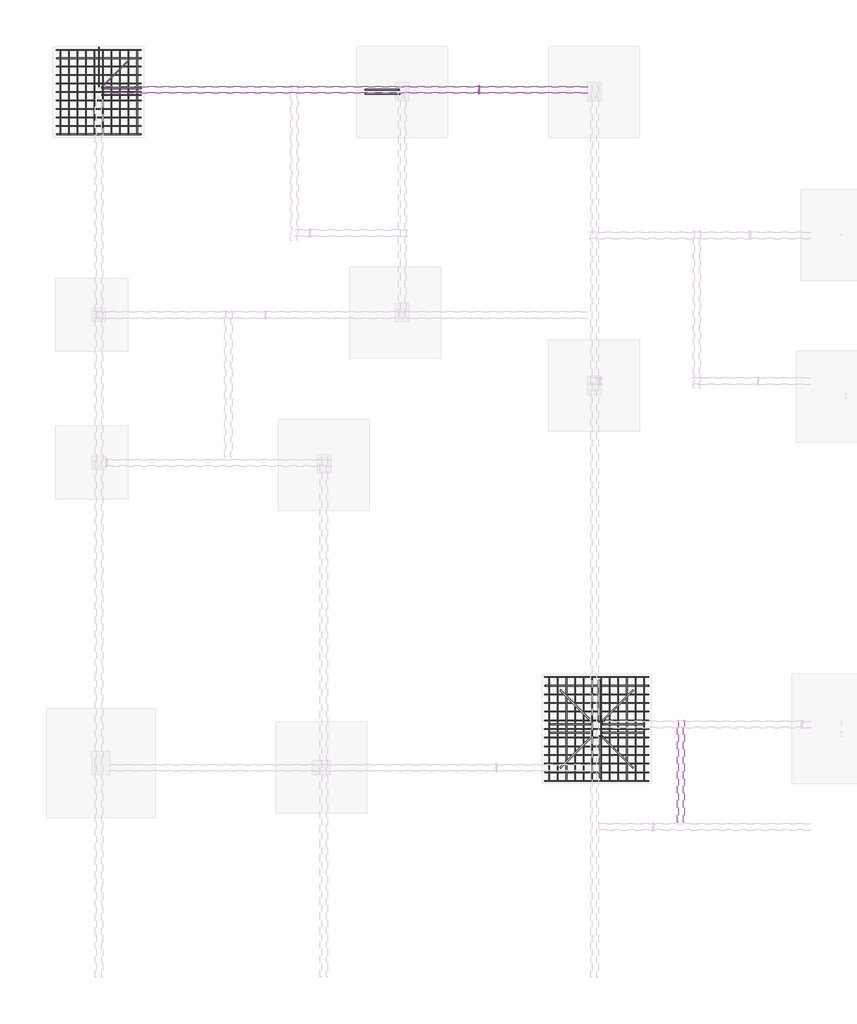
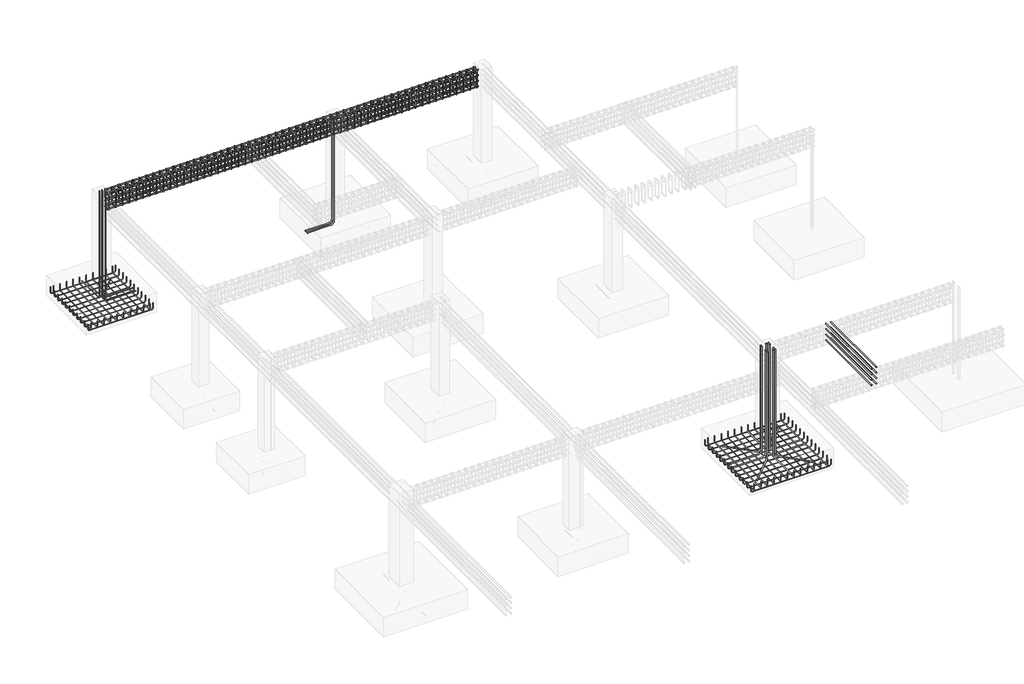
# One storey, part 7 of 10: 24 reinforcing bars.
"""IFC4 building model written with IfcOpenShell, lengths in millimetres."""

from ifc_helpers import new_model, si_unit, point, frame, origin, place, context, project, spatial, polyline, circle_curve, trimmed, segment, composite_curve, source, transform, mapped, element, save
from ifc_brep_helpers import swept_disk

model = new_model("IFC4")

# Units and contexts
model_context = context("Model", 3, world=origin())
ifc_project = project(units=[si_unit("LENGTHUNIT", "METRE", prefix="MILLI")], contexts=[model_context])

# Site, building, storey
site = spatial("IfcSite", under=ifc_project)
building = spatial("IfcBuilding", under=site)
storey = spatial("IfcBuildingStorey", under=building, Elevation=-2133.6)

# Reinforcing bars
placement = place(None, origin())
reinforcing_bar_shape = source(origin(), model_context, "Body", "SolidModel", [
    swept_disk(composite_curve([segment(polyline([(-4228.0164362, 12858.0219177, -2383.6), (-4228.0164362, 12858.0219177, -2494.1)]), True, "CONTINUOUS"), segment(trimmed(circle_curve(frame((-4262.7664362, 12858.0219177, -2494.1), z_axis=(0.0, 1.0, 0.0), x_axis=(34.75, 0.0, 0.0)), 34.75), [point((-4228.0164362, 12858.0219177, -2494.1))], [point((-4262.7664362, 12858.0219177, -2528.85))], True, "CARTESIAN"), True, "CONTINUOUS"), segment(polyline([(-4262.7664362, 12858.0219177, -2528.85), (-5607.7664362, 12858.0219177, -2528.85)]), True, "CONTINUOUS"), segment(trimmed(circle_curve(frame((-5607.7664362, 12858.0219177, -2494.1), z_axis=(0.0, 1.0, 0.0), x_axis=(0.0, 0.0, -34.75)), 34.75), [point((-5607.7664362, 12858.0219177, -2528.85))], [point((-5642.5164362, 12858.0219177, -2494.1))], True, "CARTESIAN"), True, "CONTINUOUS"), segment(polyline([(-5642.5164362, 12858.0219177, -2494.1), (-5642.5164362, 12858.0219177, -2383.6)]), True, "CONTINUOUS")], self_intersect=False), 4.75),
])
element("IfcReinforcingBar", 1, at=placement, inside=storey, context=model_context, shape_type="MappedRepresentation", body=[
    mapped(reinforcing_bar_shape, transform((0.0, 0.0, 0.0), x_axis=(1.0, 0.0, 0.0), y_axis=(0.0, 1.0, 0.0), z_axis=(0.0, 0.0, 1.0))),
    mapped(reinforcing_bar_shape, transform((0.0, -141.45, 0.0), x_axis=(1.0, 0.0, 0.0), y_axis=(0.0, 1.0, 0.0), z_axis=(0.0, 0.0, 1.0))),
    mapped(reinforcing_bar_shape, transform((0.0, -282.9, 0.0), x_axis=(1.0, 0.0, 0.0), y_axis=(0.0, 1.0, 0.0), z_axis=(0.0, 0.0, 1.0))),
    mapped(reinforcing_bar_shape, transform((0.0, -424.35, 0.0), x_axis=(1.0, 0.0, 0.0), y_axis=(0.0, 1.0, 0.0), z_axis=(0.0, 0.0, 1.0))),
    mapped(reinforcing_bar_shape, transform((0.0, -565.8, 0.0), x_axis=(1.0, 0.0, 0.0), y_axis=(0.0, 1.0, 0.0), z_axis=(0.0, 0.0, 1.0))),
    mapped(reinforcing_bar_shape, transform((0.0, -707.25, 0.0), x_axis=(1.0, 0.0, 0.0), y_axis=(0.0, 1.0, 0.0), z_axis=(0.0, 0.0, 1.0))),
    mapped(reinforcing_bar_shape, transform((0.0, -848.7, 0.0), x_axis=(1.0, 0.0, 0.0), y_axis=(0.0, 1.0, 0.0), z_axis=(0.0, 0.0, 1.0))),
    mapped(reinforcing_bar_shape, transform((0.0, -990.15, 0.0), x_axis=(1.0, 0.0, 0.0), y_axis=(0.0, 1.0, 0.0), z_axis=(0.0, 0.0, 1.0))),
    mapped(reinforcing_bar_shape, transform((0.0, -1131.6, 0.0), x_axis=(1.0, 0.0, 0.0), y_axis=(0.0, 1.0, 0.0), z_axis=(0.0, 0.0, 1.0))),
    mapped(reinforcing_bar_shape, transform((0.0, -1273.05, 0.0), x_axis=(1.0, 0.0, 0.0), y_axis=(0.0, 1.0, 0.0), z_axis=(0.0, 0.0, 1.0))),
    mapped(reinforcing_bar_shape, transform((0.0, -1414.5, 0.0), x_axis=(1.0, 0.0, 0.0), y_axis=(0.0, 1.0, 0.0), z_axis=(0.0, 0.0, 1.0))),
])
reinforcing_bar_2_shape = source(origin(), model_context, "Body", "SolidModel", [
    swept_disk(composite_curve([segment(polyline([(-4292.9743867, 11443.5219177, -2379.223371), (-4292.9743867, 11443.5219177, -2489.723371)]), True, "CONTINUOUS"), segment(trimmed(circle_curve(frame((-4292.9743867, 11478.2719177, -2489.723371), z_axis=(1.0, 0.0, 0.0), x_axis=(0.0, -34.75, 0.0)), 34.75), [point((-4292.9743867, 11443.5219177, -2489.723371))], [point((-4292.9743867, 11478.2719177, -2524.473371))], True, "CARTESIAN"), True, "CONTINUOUS"), segment(polyline([(-4292.9743867, 11478.2719177, -2524.473371), (-4292.9743867, 12823.2719177, -2524.473371)]), True, "CONTINUOUS"), segment(trimmed(circle_curve(frame((-4292.9743867, 12823.2719177, -2489.723371), z_axis=(1.0, 0.0, 0.0), x_axis=(0.0, 0.0, -34.75)), 34.75), [point((-4292.9743867, 12823.2719177, -2524.473371))], [point((-4292.9743867, 12858.0219177, -2489.723371))], True, "CARTESIAN"), True, "CONTINUOUS"), segment(polyline([(-4292.9743867, 12858.0219177, -2489.723371), (-4292.9743867, 12858.0219177, -2379.223371)]), True, "CONTINUOUS")], self_intersect=False), 4.75),
])
element("IfcReinforcingBar", 2, at=placement, inside=storey, context=model_context, shape_type="MappedRepresentation", body=[
    mapped(reinforcing_bar_2_shape, transform((0.0, 0.0, 0.0), x_axis=(1.0, 0.0, 0.0), y_axis=(0.0, 1.0, 0.0), z_axis=(0.0, 0.0, 1.0))),
    mapped(reinforcing_bar_2_shape, transform((-143.1506365, 0.0, 0.0), x_axis=(1.0, 0.0, 0.0), y_axis=(0.0, 1.0, 0.0), z_axis=(0.0, 0.0, 1.0))),
    mapped(reinforcing_bar_2_shape, transform((-286.301273, 0.0, 0.0), x_axis=(1.0, 0.0, 0.0), y_axis=(0.0, 1.0, 0.0), z_axis=(0.0, 0.0, 1.0))),
    mapped(reinforcing_bar_2_shape, transform((-429.4519095, 0.0, 0.0), x_axis=(1.0, 0.0, 0.0), y_axis=(0.0, 1.0, 0.0), z_axis=(0.0, 0.0, 1.0))),
    mapped(reinforcing_bar_2_shape, transform((-572.602546, 0.0, 0.0), x_axis=(1.0, 0.0, 0.0), y_axis=(0.0, 1.0, 0.0), z_axis=(0.0, 0.0, 1.0))),
    mapped(reinforcing_bar_2_shape, transform((-715.7531825, 0.0, 0.0), x_axis=(1.0, 0.0, 0.0), y_axis=(0.0, 1.0, 0.0), z_axis=(0.0, 0.0, 1.0))),
    mapped(reinforcing_bar_2_shape, transform((-858.903819, 0.0, 0.0), x_axis=(1.0, 0.0, 0.0), y_axis=(0.0, 1.0, 0.0), z_axis=(0.0, 0.0, 1.0))),
    mapped(reinforcing_bar_2_shape, transform((-1002.0544555, 0.0, 0.0), x_axis=(1.0, 0.0, 0.0), y_axis=(0.0, 1.0, 0.0), z_axis=(0.0, 0.0, 1.0))),
    mapped(reinforcing_bar_2_shape, transform((-1145.205092, 0.0, 0.0), x_axis=(1.0, 0.0, 0.0), y_axis=(0.0, 1.0, 0.0), z_axis=(0.0, 0.0, 1.0))),
    mapped(reinforcing_bar_2_shape, transform((-1288.3557284, 0.0, 0.0), x_axis=(1.0, 0.0, 0.0), y_axis=(0.0, 1.0, 0.0), z_axis=(0.0, 0.0, 1.0))),
])
reinforcing_bar_3_shape = source(origin(), model_context, "Body", "SolidModel", [
    swept_disk(composite_curve([segment(polyline([(4278.2835638, 2353.1839177, -2393.6), (4278.2835638, 2353.1839177, -2504.1)]), True, "CONTINUOUS"), segment(trimmed(circle_curve(frame((4243.5335638, 2353.1839177, -2504.1), z_axis=(0.0, 1.0, 0.0), x_axis=(34.75, 0.0, 0.0)), 34.75), [point((4278.2835638, 2353.1839177, -2504.1))], [point((4243.5335638, 2353.1839177, -2538.85))], True, "CARTESIAN"), True, "CONTINUOUS"), segment(polyline([(4243.5335638, 2353.1839177, -2538.85), (2573.7335638, 2353.1839177, -2538.85)]), True, "CONTINUOUS"), segment(trimmed(circle_curve(frame((2573.7335638, 2353.1839177, -2504.1), z_axis=(0.0, 1.0, 0.0), x_axis=(0.0, 0.0, -34.75)), 34.75), [point((2573.7335638, 2353.1839177, -2538.85))], [point((2538.9835638, 2353.1839177, -2504.1))], True, "CARTESIAN"), True, "CONTINUOUS"), segment(polyline([(2538.9835638, 2353.1839177, -2504.1), (2538.9835638, 2353.1839177, -2393.6)]), True, "CONTINUOUS")], self_intersect=False), 4.75),
])
element("IfcReinforcingBar", 3, at=placement, inside=storey, context=model_context, shape_type="MappedRepresentation", body=[
    mapped(reinforcing_bar_3_shape, transform((0.0, 0.0, 0.0), x_axis=(1.0, 0.0, 0.0), y_axis=(0.0, 1.0, 0.0), z_axis=(0.0, 0.0, 1.0))),
    mapped(reinforcing_bar_3_shape, transform((0.0, -144.9416667, 0.0), x_axis=(1.0, 0.0, 0.0), y_axis=(0.0, 1.0, 0.0), z_axis=(0.0, 0.0, 1.0))),
    mapped(reinforcing_bar_3_shape, transform((0.0, -289.8833333, 0.0), x_axis=(1.0, 0.0, 0.0), y_axis=(0.0, 1.0, 0.0), z_axis=(0.0, 0.0, 1.0))),
    mapped(reinforcing_bar_3_shape, transform((0.0, -434.825, 0.0), x_axis=(1.0, 0.0, 0.0), y_axis=(0.0, 1.0, 0.0), z_axis=(0.0, 0.0, 1.0))),
    mapped(reinforcing_bar_3_shape, transform((0.0, -579.7666667, 0.0), x_axis=(1.0, 0.0, 0.0), y_axis=(0.0, 1.0, 0.0), z_axis=(0.0, 0.0, 1.0))),
    mapped(reinforcing_bar_3_shape, transform((0.0, -724.7083333, 0.0), x_axis=(1.0, 0.0, 0.0), y_axis=(0.0, 1.0, 0.0), z_axis=(0.0, 0.0, 1.0))),
    mapped(reinforcing_bar_3_shape, transform((0.0, -869.65, 0.0), x_axis=(1.0, 0.0, 0.0), y_axis=(0.0, 1.0, 0.0), z_axis=(0.0, 0.0, 1.0))),
    mapped(reinforcing_bar_3_shape, transform((0.0, -1014.5916667, 0.0), x_axis=(1.0, 0.0, 0.0), y_axis=(0.0, 1.0, 0.0), z_axis=(0.0, 0.0, 1.0))),
    mapped(reinforcing_bar_3_shape, transform((0.0, -1159.5333333, 0.0), x_axis=(1.0, 0.0, 0.0), y_axis=(0.0, 1.0, 0.0), z_axis=(0.0, 0.0, 1.0))),
    mapped(reinforcing_bar_3_shape, transform((0.0, -1304.475, 0.0), x_axis=(1.0, 0.0, 0.0), y_axis=(0.0, 1.0, 0.0), z_axis=(0.0, 0.0, 1.0))),
    mapped(reinforcing_bar_3_shape, transform((0.0, -1449.4166667, 0.0), x_axis=(1.0, 0.0, 0.0), y_axis=(0.0, 1.0, 0.0), z_axis=(0.0, 0.0, 1.0))),
    mapped(reinforcing_bar_3_shape, transform((0.0, -1594.3583333, 0.0), x_axis=(1.0, 0.0, 0.0), y_axis=(0.0, 1.0, 0.0), z_axis=(0.0, 0.0, 1.0))),
    mapped(reinforcing_bar_3_shape, transform((0.0, -1739.3, 0.0), x_axis=(1.0, 0.0, 0.0), y_axis=(0.0, 1.0, 0.0), z_axis=(0.0, 0.0, 1.0))),
])
reinforcing_bar_4_shape = source(origin(), model_context, "Body", "SolidModel", [
    swept_disk(composite_curve([segment(polyline([(4203.3256133, 613.8839177, -2379.223371), (4203.3256133, 613.8839177, -2489.723371)]), True, "CONTINUOUS"), segment(trimmed(circle_curve(frame((4203.3256133, 648.6339177, -2489.723371), z_axis=(1.0, 0.0, 0.0), x_axis=(0.0, -34.75, 0.0)), 34.75), [point((4203.3256133, 613.8839177, -2489.723371))], [point((4203.3256133, 648.6339177, -2524.473371))], True, "CARTESIAN"), True, "CONTINUOUS"), segment(polyline([(4203.3256133, 648.6339177, -2524.473371), (4203.3256133, 2318.4339177, -2524.473371)]), True, "CONTINUOUS"), segment(trimmed(circle_curve(frame((4203.3256133, 2318.4339177, -2489.723371), z_axis=(1.0, 0.0, 0.0), x_axis=(0.0, 0.0, -34.75)), 34.75), [point((4203.3256133, 2318.4339177, -2524.473371))], [point((4203.3256133, 2353.1839177, -2489.723371))], True, "CARTESIAN"), True, "CONTINUOUS"), segment(polyline([(4203.3256133, 2353.1839177, -2489.723371), (4203.3256133, 2353.1839177, -2379.223371)]), True, "CONTINUOUS")], self_intersect=False), 4.75),
])
element("IfcReinforcingBar", 4, at=placement, inside=storey, context=model_context, shape_type="MappedRepresentation", body=[
    mapped(reinforcing_bar_4_shape, transform((0.0, 0.0, 0.0), x_axis=(1.0, 0.0, 0.0), y_axis=(0.0, 1.0, 0.0), z_axis=(0.0, 0.0, 1.0))),
    mapped(reinforcing_bar_4_shape, transform((-144.8323389, 0.0, 0.0), x_axis=(1.0, 0.0, 0.0), y_axis=(0.0, 1.0, 0.0), z_axis=(0.0, 0.0, 1.0))),
    mapped(reinforcing_bar_4_shape, transform((-289.6646779, 0.0, 0.0), x_axis=(1.0, 0.0, 0.0), y_axis=(0.0, 1.0, 0.0), z_axis=(0.0, 0.0, 1.0))),
    mapped(reinforcing_bar_4_shape, transform((-434.4970168, 0.0, 0.0), x_axis=(1.0, 0.0, 0.0), y_axis=(0.0, 1.0, 0.0), z_axis=(0.0, 0.0, 1.0))),
    mapped(reinforcing_bar_4_shape, transform((-579.3293558, 0.0, 0.0), x_axis=(1.0, 0.0, 0.0), y_axis=(0.0, 1.0, 0.0), z_axis=(0.0, 0.0, 1.0))),
    mapped(reinforcing_bar_4_shape, transform((-724.1616947, 0.0, 0.0), x_axis=(1.0, 0.0, 0.0), y_axis=(0.0, 1.0, 0.0), z_axis=(0.0, 0.0, 1.0))),
    mapped(reinforcing_bar_4_shape, transform((-868.9940337, 0.0, 0.0), x_axis=(1.0, 0.0, 0.0), y_axis=(0.0, 1.0, 0.0), z_axis=(0.0, 0.0, 1.0))),
    mapped(reinforcing_bar_4_shape, transform((-1013.8263726, 0.0, 0.0), x_axis=(1.0, 0.0, 0.0), y_axis=(0.0, 1.0, 0.0), z_axis=(0.0, 0.0, 1.0))),
    mapped(reinforcing_bar_4_shape, transform((-1158.6587116, 0.0, 0.0), x_axis=(1.0, 0.0, 0.0), y_axis=(0.0, 1.0, 0.0), z_axis=(0.0, 0.0, 1.0))),
    mapped(reinforcing_bar_4_shape, transform((-1303.4910505, 0.0, 0.0), x_axis=(1.0, 0.0, 0.0), y_axis=(0.0, 1.0, 0.0), z_axis=(0.0, 0.0, 1.0))),
    mapped(reinforcing_bar_4_shape, transform((-1448.3233895, 0.0, 0.0), x_axis=(1.0, 0.0, 0.0), y_axis=(0.0, 1.0, 0.0), z_axis=(0.0, 0.0, 1.0))),
    mapped(reinforcing_bar_4_shape, transform((-1593.1557284, 0.0, 0.0), x_axis=(1.0, 0.0, 0.0), y_axis=(0.0, 1.0, 0.0), z_axis=(0.0, 0.0, 1.0))),
])
element("IfcReinforcingBar", 5, at=placement, inside=storey, context=model_context, shape_type="SolidModel", body=[
    swept_disk(composite_curve([segment(polyline([(103.3335638, 12191.9552961, -40.0), (103.3335638, 12191.9552961, -2426.55)]), True, "CONTINUOUS"), segment(trimmed(circle_curve(frame((36.2835638, 12191.9552961, -2426.55), z_axis=(0.0, 1.0, 0.0), x_axis=(67.04999999999998, 0.0, 0.0)), 67.05), [point((103.3335638, 12191.9552961, -2426.55))], [point((36.2835638, 12191.9552961, -2493.6))], True, "CARTESIAN"), True, "CONTINUOUS"), segment(polyline([(36.2835638, 12191.9552961, -2493.6), (-476.6664362, 12191.9552961, -2493.6)]), True, "CONTINUOUS")], self_intersect=False), 9.55),
])
element("IfcReinforcingBar", 6, at=placement, inside=storey, context=model_context, shape_type="SolidModel", body=[
    swept_disk(composite_curve([segment(polyline([(103.3335638, 12124.8170998, -40.0), (103.3335638, 12124.8170998, -2426.55)]), True, "CONTINUOUS"), segment(trimmed(circle_curve(frame((36.2835638, 12124.8170998, -2426.55), z_axis=(0.0, 1.0, 0.0), x_axis=(67.04999999999998, 0.0, 0.0)), 67.05), [point((103.3335638, 12124.8170998, -2426.55))], [point((36.2835638, 12124.8170998, -2493.6))], True, "CARTESIAN"), True, "CONTINUOUS"), segment(polyline([(36.2835638, 12124.8170998, -2493.6), (-476.6664362, 12124.8170998, -2493.6)]), True, "CONTINUOUS")], self_intersect=False), 9.55),
])
element("IfcReinforcingBar", 7, at=placement, inside=storey, context=model_context, shape_type="SolidModel", body=[
    swept_disk(composite_curve([segment(polyline([(-4880.7190942, 12237.3982446, -40.0), (-4880.7190942, 12237.3982446, -2478.85)]), True, "CONTINUOUS"), segment(trimmed(circle_curve(frame((-4856.1471335, 12261.9702053, -2478.85), z_axis=(0.7071067811865476, -0.7071067811865475, 0.0), x_axis=(-24.57196070000009, -24.57196069999918, 0.0)), 34.75), [point((-4880.7190942, 12237.3982446, -2478.85))], [point((-4856.1471335, 12261.9702053, -2513.6))], True, "CARTESIAN"), True, "CONTINUOUS"), segment(polyline([(-4856.1471335, 12261.9702053, -2513.6), (-4415.8298614, 12702.2874774, -2513.6)]), True, "CONTINUOUS")], self_intersect=False), 4.75),
])
reinforcing_bar_5_shape = source(origin(), model_context, "Body", "SolidModel", [
    swept_disk(composite_curve([segment(polyline([(-4880.7190942, 12214.7595351, -40.0), (-4880.7190942, 12214.7595351, -2478.85)]), True, "CONTINUOUS"), segment(trimmed(circle_curve(frame((-4845.9690942, 12214.7595351, -2478.85), z_axis=(0.0, -1.0, 0.0), x_axis=(-34.75, 0.0, 0.0)), 34.75), [point((-4880.7190942, 12214.7595351, -2478.85))], [point((-4845.9690942, 12214.7595351, -2513.6))], True, "CARTESIAN"), True, "CONTINUOUS"), segment(polyline([(-4845.9690942, 12214.7595351, -2513.6), (-4223.2664362, 12214.7595351, -2513.6)]), True, "CONTINUOUS")], self_intersect=False), 4.75),
])
element("IfcReinforcingBar", 8, at=placement, inside=storey, context=model_context, shape_type="MappedRepresentation", body=[
    mapped(reinforcing_bar_5_shape, transform((0.0, 0.0, 0.0), x_axis=(1.0, 0.0, 0.0), y_axis=(0.0, 1.0, 0.0), z_axis=(0.0, 0.0, 1.0))),
    mapped(reinforcing_bar_5_shape, transform((0.0, -114.7595265, 0.0), x_axis=(1.0, 0.0, 0.0), y_axis=(0.0, 1.0, 0.0), z_axis=(0.0, 0.0, 1.0))),
])
element("IfcReinforcingBar", 9, at=placement, inside=storey, context=model_context, shape_type="SolidModel", body=[
    swept_disk(composite_curve([segment(polyline([(-4935.2664362, 12242.3982446, -40.0), (-4935.2664362, 12242.3982446, -2478.85)]), True, "CONTINUOUS"), segment(trimmed(circle_curve(frame((-4935.2664362, 12277.1482446, -2478.85), z_axis=(1.0, 0.0, 0.0), x_axis=(0.0, -34.75, 0.0)), 34.75), [point((-4935.2664362, 12242.3982446, -2478.85))], [point((-4935.2664362, 12277.1482446, -2513.6))], True, "CARTESIAN"), True, "CONTINUOUS"), segment(polyline([(-4935.2664362, 12277.1482446, -2513.6), (-4935.2664362, 12899.8509026, -2513.6)]), True, "CONTINUOUS")], self_intersect=False), 4.75),
])
element("IfcReinforcingBar", 10, at=placement, inside=storey, context=model_context, shape_type="SolidModel", body=[
    swept_disk(composite_curve([segment(polyline([(3323.3335638, 1607.8172961, -40.0), (3323.3335638, 1607.8172961, -2426.55)]), True, "CONTINUOUS"), segment(trimmed(circle_curve(frame((3275.9220542, 1655.2288058, -2426.55), z_axis=(0.707106781186552, 0.7071067811865431, 0.0), x_axis=(47.411509600000045, -47.4115096999999, 0.0)), 67.05), [point((3323.3335638, 1607.8172961, -2426.55))], [point((3275.9220542, 1655.2288058, -2493.6))], True, "CARTESIAN"), True, "CONTINUOUS"), segment(polyline([(3275.9220542, 1655.2288058, -2493.6), (2798.9116308, 2132.2392292, -2493.6)]), True, "CONTINUOUS")], self_intersect=False), 9.55),
])
element("IfcReinforcingBar", 11, at=placement, inside=storey, context=model_context, shape_type="SolidModel", body=[
    swept_disk(composite_curve([segment(polyline([(3495.0335638, 1607.8172961, -40.0), (3495.0335638, 1607.8172961, -2426.55)]), True, "CONTINUOUS"), segment(trimmed(circle_curve(frame((3542.4450735, 1655.2288058, -2426.55), z_axis=(0.7071067811865519, -0.7071067811865431, 0.0), x_axis=(-47.4115096999999, -47.4115096999999, 0.0)), 67.05), [point((3495.0335638, 1607.8172961, -2426.55))], [point((3542.4450735, 1655.2288058, -2493.6))], True, "CARTESIAN"), True, "CONTINUOUS"), segment(polyline([(3542.4450735, 1655.2288058, -2493.6), (4019.4554969, 2132.2392292, -2493.6)]), True, "CONTINUOUS")], self_intersect=False), 9.55),
])
element("IfcReinforcingBar", 12, at=placement, inside=storey, context=model_context, shape_type="SolidModel", body=[
    swept_disk(composite_curve([segment(polyline([(3323.3335638, 1359.2505393, -40.0), (3323.3335638, 1359.2505393, -2426.55)]), True, "CONTINUOUS"), segment(trimmed(circle_curve(frame((3275.9220542, 1311.8390296, -2426.55), z_axis=(-0.7071067811865519, 0.7071067811865431, 0.0), x_axis=(47.411509600000045, 47.4115096999999, 0.0)), 67.05), [point((3323.3335638, 1359.2505393, -2426.55))], [point((3275.9220542, 1311.8390296, -2493.6))], True, "CARTESIAN"), True, "CONTINUOUS"), segment(polyline([(3275.9220542, 1311.8390296, -2493.6), (2798.9116308, 834.8286062, -2493.6)]), True, "CONTINUOUS")], self_intersect=False), 9.55),
])
element("IfcReinforcingBar", 13, at=placement, inside=storey, context=model_context, shape_type="SolidModel", body=[
    swept_disk(composite_curve([segment(polyline([(3495.0335638, 1359.2505393, -40.0), (3495.0335638, 1359.2505393, -2426.55)]), True, "CONTINUOUS"), segment(trimmed(circle_curve(frame((3542.4450735, 1311.8390296, -2426.55), z_axis=(-0.7071067811865519, -0.7071067811865431, 0.0), x_axis=(-47.4115096999999, 47.4115096999999, 0.0)), 67.05), [point((3495.0335638, 1359.2505393, -2426.55))], [point((3542.4450735, 1311.8390296, -2493.6))], True, "CARTESIAN"), True, "CONTINUOUS"), segment(polyline([(3542.4450735, 1311.8390296, -2493.6), (4019.4554969, 834.8286062, -2493.6)]), True, "CONTINUOUS")], self_intersect=False), 9.55),
])
element("IfcReinforcingBar", 14, at=placement, inside=storey, context=model_context, shape_type="SolidModel", body=[
    swept_disk(composite_curve([segment(polyline([(3448.4194855, 1607.8172961, -40.0), (3448.4194855, 1607.8172961, -2426.55)]), True, "CONTINUOUS"), segment(trimmed(circle_curve(frame((3448.4194855, 1674.8672961, -2426.55), z_axis=(1.0, 0.0, 0.0), x_axis=(0.0, -67.04999999999995, 0.0)), 67.05), [point((3448.4194855, 1607.8172961, -2426.55))], [point((3448.4194855, 1674.8672961, -2493.6))], True, "CARTESIAN"), True, "CONTINUOUS"), segment(polyline([(3448.4194855, 1674.8672961, -2493.6), (3448.4194855, 2302.1172961, -2493.6)]), True, "CONTINUOUS")], self_intersect=False), 9.55),
])
element("IfcReinforcingBar", 15, at=placement, inside=storey, context=model_context, shape_type="SolidModel", body=[
    swept_disk(composite_curve([segment(polyline([(3458.4194855, 1359.2505393, -40.0), (3458.4194855, 1359.2505393, -2426.55)]), True, "CONTINUOUS"), segment(trimmed(circle_curve(frame((3458.4194855, 1292.2005393, -2426.55), z_axis=(-1.0, 0.0, 0.0), x_axis=(0.0, 67.04999999999995, 0.0)), 67.05), [point((3458.4194855, 1359.2505393, -2426.55))], [point((3458.4194855, 1292.2005393, -2493.6))], True, "CARTESIAN"), True, "CONTINUOUS"), segment(polyline([(3458.4194855, 1292.2005393, -2493.6), (3458.4194855, 664.9505393, -2493.6)]), True, "CONTINUOUS")], self_intersect=False), 9.55),
])
element("IfcReinforcingBar", 16, at=placement, inside=storey, context=model_context, shape_type="SolidModel", body=[
    swept_disk(composite_curve([segment(polyline([(3323.3335638, 1562.8172961, -40.0), (3323.3335638, 1562.8172961, -2426.55)]), True, "CONTINUOUS"), segment(trimmed(circle_curve(frame((3256.2835638, 1562.8172961, -2426.55), z_axis=(0.0, 1.0, 0.0), x_axis=(67.04999999999973, 0.0, 0.0)), 67.05), [point((3323.3335638, 1562.8172961, -2426.55))], [point((3256.2835638, 1562.8172961, -2493.6))], True, "CARTESIAN"), True, "CONTINUOUS"), segment(polyline([(3256.2835638, 1562.8172961, -2493.6), (2629.0335638, 1562.8172961, -2493.6)]), True, "CONTINUOUS")], self_intersect=False), 9.55),
])
element("IfcReinforcingBar", 17, at=placement, inside=storey, context=model_context, shape_type="SolidModel", body=[
    swept_disk(composite_curve([segment(polyline([(3323.3335638, 1419.4790998, -40.0), (3323.3335638, 1419.4790998, -2426.55)]), True, "CONTINUOUS"), segment(trimmed(circle_curve(frame((3256.2835638, 1419.4790998, -2426.55), z_axis=(0.0, 1.0, 0.0), x_axis=(67.04999999999973, 0.0, 0.0)), 67.05), [point((3323.3335638, 1419.4790998, -2426.55))], [point((3256.2835638, 1419.4790998, -2493.6))], True, "CARTESIAN"), True, "CONTINUOUS"), segment(polyline([(3256.2835638, 1419.4790998, -2493.6), (2629.0335638, 1419.4790998, -2493.6)]), True, "CONTINUOUS")], self_intersect=False), 9.55),
])
element("IfcReinforcingBar", 18, at=placement, inside=storey, context=model_context, shape_type="SolidModel", body=[
    swept_disk(composite_curve([segment(polyline([(3495.0335638, 1562.8172961, -40.0), (3495.0335638, 1562.8172961, -2426.55)]), True, "CONTINUOUS"), segment(trimmed(circle_curve(frame((3562.0835638, 1562.8172961, -2426.55), z_axis=(0.0, -1.0, 0.0), x_axis=(-67.04999999999973, 0.0, 0.0)), 67.05), [point((3495.0335638, 1562.8172961, -2426.55))], [point((3562.0835638, 1562.8172961, -2493.6))], True, "CARTESIAN"), True, "CONTINUOUS"), segment(polyline([(3562.0835638, 1562.8172961, -2493.6), (4189.3335638, 1562.8172961, -2493.6)]), True, "CONTINUOUS")], self_intersect=False), 9.55),
])
element("IfcReinforcingBar", 19, at=placement, inside=storey, context=model_context, shape_type="SolidModel", body=[
    swept_disk(composite_curve([segment(polyline([(3495.0335638, 1419.4790998, -40.0), (3495.0335638, 1419.4790998, -2426.55)]), True, "CONTINUOUS"), segment(trimmed(circle_curve(frame((3562.0835638, 1419.4790998, -2426.55), z_axis=(0.0, -1.0, 0.0), x_axis=(-67.04999999999973, 0.0, 0.0)), 67.05), [point((3495.0335638, 1419.4790998, -2426.55))], [point((3562.0835638, 1419.4790998, -2493.6))], True, "CARTESIAN"), True, "CONTINUOUS"), segment(polyline([(3562.0835638, 1419.4790998, -2493.6), (4189.3335638, 1419.4790998, -2493.6)]), True, "CONTINUOUS")], self_intersect=False), 9.55),
])
reinforcing_bar_6_shape = source(origin(), model_context, "Body", "SolidModel", [
    swept_disk(composite_curve([segment(polyline([(-4794.7605396, 12218.9786993, -109.4049959), (-4794.7605396, 12161.5728105, -51.9991072)]), True, "CONTINUOUS"), segment(trimmed(circle_curve(frame((-4794.7605396, 12144.0719177, -69.5), z_axis=(1.0, 0.0, 0.0), x_axis=(0.0, 17.500892800000656, 17.500892800000003)), 24.75), [point((-4794.7605396, 12161.5728105, -51.9991072))], [point((-4794.7605396, 12119.3219177, -69.5))], True, "CARTESIAN"), True, "CONTINUOUS"), segment(polyline([(-4794.7605396, 12119.3219177, -69.5), (-4794.7605396, 12119.3219177, -430.5)]), True, "CONTINUOUS"), segment(trimmed(circle_curve(frame((-4794.7605396, 12144.0719177, -430.5), z_axis=(1.0, 0.0, 0.0), x_axis=(0.0, -24.75, 0.0)), 24.75), [point((-4794.7605396, 12119.3219177, -430.5))], [point((-4794.7605396, 12144.0719177, -455.25))], True, "CARTESIAN"), True, "CONTINUOUS"), segment(polyline([(-4794.7605396, 12144.0719177, -455.25), (-4794.7605396, 12233.6719177, -455.25)]), True, "CONTINUOUS"), segment(trimmed(circle_curve(frame((-4795.3331634, 12233.6719177, -430.5066251), z_axis=(0.9997323196529888, 0.0, 0.02313631434032496), x_axis=(0.5726237999997466, 0.0, -24.743374899999992)), 24.75), [point((-4794.7605396, 12233.6719177, -455.25))], [point((-4795.3331634, 12258.4219177, -430.5066251))], True, "CARTESIAN"), True, "CONTINUOUS"), segment(polyline([(-4795.3331634, 12258.4219177, -430.5066251), (-4803.6879158, 12258.4219177, -69.4933749)]), True, "CONTINUOUS"), segment(trimmed(circle_curve(frame((-4803.6879158, 12233.6719177, -69.4933749), z_axis=(0.9997323196529888, 0.0, 0.02313631434032496), x_axis=(0.0, 24.75, 0.0)), 24.75), [point((-4803.6879158, 12258.4219177, -69.4933749))], [point((-4804.2605396, 12233.6719177, -44.75))], True, "CARTESIAN"), True, "CONTINUOUS"), segment(polyline([(-4804.2605396, 12233.6719177, -44.75), (-4804.2605396, 12144.0719177, -44.75)]), True, "CONTINUOUS"), segment(trimmed(circle_curve(frame((-4804.2605396, 12144.0719177, -69.5), z_axis=(1.0, 0.0, 0.0), x_axis=(0.0, 0.0, 24.75)), 24.75), [point((-4804.2605396, 12144.0719177, -44.75))], [point((-4804.2605396, 12126.5710249, -87.0008928))], True, "CARTESIAN"), True, "CONTINUOUS"), segment(polyline([(-4804.2605396, 12126.5710249, -87.0008928), (-4804.2605396, 12183.9769136, -144.4067815)]), True, "CONTINUOUS")], self_intersect=False), 4.75),
])
element("IfcReinforcingBar", 20, at=placement, inside=storey, context=model_context, shape_type="MappedRepresentation", body=[
    mapped(reinforcing_bar_6_shape, transform((0.0, 0.0, 0.0), x_axis=(1.0, 0.0, 0.0), y_axis=(0.0, 1.0, 0.0), z_axis=(0.0, 0.0, 1.0))),
    mapped(reinforcing_bar_6_shape, transform((148.4199023, 0.0, 0.0), x_axis=(1.0, 0.0, 0.0), y_axis=(0.0, 1.0, 0.0), z_axis=(0.0, 0.0, 1.0))),
    mapped(reinforcing_bar_6_shape, transform((296.8398046, 0.0, 0.0), x_axis=(1.0, 0.0, 0.0), y_axis=(0.0, 1.0, 0.0), z_axis=(0.0, 0.0, 1.0))),
    mapped(reinforcing_bar_6_shape, transform((445.2597069, 0.0, 0.0), x_axis=(1.0, 0.0, 0.0), y_axis=(0.0, 1.0, 0.0), z_axis=(0.0, 0.0, 1.0))),
    mapped(reinforcing_bar_6_shape, transform((593.6796092, 0.0, 0.0), x_axis=(1.0, 0.0, 0.0), y_axis=(0.0, 1.0, 0.0), z_axis=(0.0, 0.0, 1.0))),
    mapped(reinforcing_bar_6_shape, transform((742.0995115, 0.0, 0.0), x_axis=(1.0, 0.0, 0.0), y_axis=(0.0, 1.0, 0.0), z_axis=(0.0, 0.0, 1.0))),
    mapped(reinforcing_bar_6_shape, transform((890.5194138, 0.0, 0.0), x_axis=(1.0, 0.0, 0.0), y_axis=(0.0, 1.0, 0.0), z_axis=(0.0, 0.0, 1.0))),
    mapped(reinforcing_bar_6_shape, transform((1038.9393161, 0.0, 0.0), x_axis=(1.0, 0.0, 0.0), y_axis=(0.0, 1.0, 0.0), z_axis=(0.0, 0.0, 1.0))),
    mapped(reinforcing_bar_6_shape, transform((1187.3592184, 0.0, 0.0), x_axis=(1.0, 0.0, 0.0), y_axis=(0.0, 1.0, 0.0), z_axis=(0.0, 0.0, 1.0))),
    mapped(reinforcing_bar_6_shape, transform((1335.7791207, 0.0, 0.0), x_axis=(1.0, 0.0, 0.0), y_axis=(0.0, 1.0, 0.0), z_axis=(0.0, 0.0, 1.0))),
    mapped(reinforcing_bar_6_shape, transform((1484.199023, 0.0, 0.0), x_axis=(1.0, 0.0, 0.0), y_axis=(0.0, 1.0, 0.0), z_axis=(0.0, 0.0, 1.0))),
    mapped(reinforcing_bar_6_shape, transform((1632.6189253, 0.0, 0.0), x_axis=(1.0, 0.0, 0.0), y_axis=(0.0, 1.0, 0.0), z_axis=(0.0, 0.0, 1.0))),
    mapped(reinforcing_bar_6_shape, transform((1781.0388275, 0.0, 0.0), x_axis=(1.0, 0.0, 0.0), y_axis=(0.0, 1.0, 0.0), z_axis=(0.0, 0.0, 1.0))),
    mapped(reinforcing_bar_6_shape, transform((1929.4587298, 0.0, 0.0), x_axis=(1.0, 0.0, 0.0), y_axis=(0.0, 1.0, 0.0), z_axis=(0.0, 0.0, 1.0))),
    mapped(reinforcing_bar_6_shape, transform((2077.8786321, 0.0, 0.0), x_axis=(1.0, 0.0, 0.0), y_axis=(0.0, 1.0, 0.0), z_axis=(0.0, 0.0, 1.0))),
    mapped(reinforcing_bar_6_shape, transform((2226.2985344, 0.0, 0.0), x_axis=(1.0, 0.0, 0.0), y_axis=(0.0, 1.0, 0.0), z_axis=(0.0, 0.0, 1.0))),
    mapped(reinforcing_bar_6_shape, transform((2374.7184367, 0.0, 0.0), x_axis=(1.0, 0.0, 0.0), y_axis=(0.0, 1.0, 0.0), z_axis=(0.0, 0.0, 1.0))),
    mapped(reinforcing_bar_6_shape, transform((2523.138339, 0.0, 0.0), x_axis=(1.0, 0.0, 0.0), y_axis=(0.0, 1.0, 0.0), z_axis=(0.0, 0.0, 1.0))),
    mapped(reinforcing_bar_6_shape, transform((2671.5582413, 0.0, 0.0), x_axis=(1.0, 0.0, 0.0), y_axis=(0.0, 1.0, 0.0), z_axis=(0.0, 0.0, 1.0))),
    mapped(reinforcing_bar_6_shape, transform((2819.9781436, 0.0, 0.0), x_axis=(1.0, 0.0, 0.0), y_axis=(0.0, 1.0, 0.0), z_axis=(0.0, 0.0, 1.0))),
    mapped(reinforcing_bar_6_shape, transform((2968.3980459, 0.0, 0.0), x_axis=(1.0, 0.0, 0.0), y_axis=(0.0, 1.0, 0.0), z_axis=(0.0, 0.0, 1.0))),
    mapped(reinforcing_bar_6_shape, transform((3116.8179482, 0.0, 0.0), x_axis=(1.0, 0.0, 0.0), y_axis=(0.0, 1.0, 0.0), z_axis=(0.0, 0.0, 1.0))),
    mapped(reinforcing_bar_6_shape, transform((3265.2378505, 0.0, 0.0), x_axis=(1.0, 0.0, 0.0), y_axis=(0.0, 1.0, 0.0), z_axis=(0.0, 0.0, 1.0))),
    mapped(reinforcing_bar_6_shape, transform((3413.6577528, 0.0, 0.0), x_axis=(1.0, 0.0, 0.0), y_axis=(0.0, 1.0, 0.0), z_axis=(0.0, 0.0, 1.0))),
    mapped(reinforcing_bar_6_shape, transform((3562.0776551, 0.0, 0.0), x_axis=(1.0, 0.0, 0.0), y_axis=(0.0, 1.0, 0.0), z_axis=(0.0, 0.0, 1.0))),
    mapped(reinforcing_bar_6_shape, transform((3710.4975574, 0.0, 0.0), x_axis=(1.0, 0.0, 0.0), y_axis=(0.0, 1.0, 0.0), z_axis=(0.0, 0.0, 1.0))),
    mapped(reinforcing_bar_6_shape, transform((3858.9174597, 0.0, 0.0), x_axis=(1.0, 0.0, 0.0), y_axis=(0.0, 1.0, 0.0), z_axis=(0.0, 0.0, 1.0))),
    mapped(reinforcing_bar_6_shape, transform((4007.337362, 0.0, 0.0), x_axis=(1.0, 0.0, 0.0), y_axis=(0.0, 1.0, 0.0), z_axis=(0.0, 0.0, 1.0))),
    mapped(reinforcing_bar_6_shape, transform((4155.7572643, 0.0, 0.0), x_axis=(1.0, 0.0, 0.0), y_axis=(0.0, 1.0, 0.0), z_axis=(0.0, 0.0, 1.0))),
    mapped(reinforcing_bar_6_shape, transform((4304.1771666, 0.0, 0.0), x_axis=(1.0, 0.0, 0.0), y_axis=(0.0, 1.0, 0.0), z_axis=(0.0, 0.0, 1.0))),
    mapped(reinforcing_bar_6_shape, transform((4452.5970689, 0.0, 0.0), x_axis=(1.0, 0.0, 0.0), y_axis=(0.0, 1.0, 0.0), z_axis=(0.0, 0.0, 1.0))),
    mapped(reinforcing_bar_6_shape, transform((4601.0169712, 0.0, 0.0), x_axis=(1.0, 0.0, 0.0), y_axis=(0.0, 1.0, 0.0), z_axis=(0.0, 0.0, 1.0))),
    mapped(reinforcing_bar_6_shape, transform((4749.4368735, 0.0, 0.0), x_axis=(1.0, 0.0, 0.0), y_axis=(0.0, 1.0, 0.0), z_axis=(0.0, 0.0, 1.0))),
    mapped(reinforcing_bar_6_shape, transform((4897.8567758, 0.0, 0.0), x_axis=(1.0, 0.0, 0.0), y_axis=(0.0, 1.0, 0.0), z_axis=(0.0, 0.0, 1.0))),
    mapped(reinforcing_bar_6_shape, transform((5046.276678, 0.0, 0.0), x_axis=(1.0, 0.0, 0.0), y_axis=(0.0, 1.0, 0.0), z_axis=(0.0, 0.0, 1.0))),
    mapped(reinforcing_bar_6_shape, transform((5194.6965803, 0.0, 0.0), x_axis=(1.0, 0.0, 0.0), y_axis=(0.0, 1.0, 0.0), z_axis=(0.0, 0.0, 1.0))),
    mapped(reinforcing_bar_6_shape, transform((5343.1164826, 0.0, 0.0), x_axis=(1.0, 0.0, 0.0), y_axis=(0.0, 1.0, 0.0), z_axis=(0.0, 0.0, 1.0))),
    mapped(reinforcing_bar_6_shape, transform((5491.5363849, 0.0, 0.0), x_axis=(1.0, 0.0, 0.0), y_axis=(0.0, 1.0, 0.0), z_axis=(0.0, 0.0, 1.0))),
    mapped(reinforcing_bar_6_shape, transform((5639.9562872, 0.0, 0.0), x_axis=(1.0, 0.0, 0.0), y_axis=(0.0, 1.0, 0.0), z_axis=(0.0, 0.0, 1.0))),
    mapped(reinforcing_bar_6_shape, transform((5788.3761895, 0.0, 0.0), x_axis=(1.0, 0.0, 0.0), y_axis=(0.0, 1.0, 0.0), z_axis=(0.0, 0.0, 1.0))),
    mapped(reinforcing_bar_6_shape, transform((5936.7960918, 0.0, 0.0), x_axis=(1.0, 0.0, 0.0), y_axis=(0.0, 1.0, 0.0), z_axis=(0.0, 0.0, 1.0))),
    mapped(reinforcing_bar_6_shape, transform((6085.2159941, 0.0, 0.0), x_axis=(1.0, 0.0, 0.0), y_axis=(0.0, 1.0, 0.0), z_axis=(0.0, 0.0, 1.0))),
    mapped(reinforcing_bar_6_shape, transform((6233.6358964, 0.0, 0.0), x_axis=(1.0, 0.0, 0.0), y_axis=(0.0, 1.0, 0.0), z_axis=(0.0, 0.0, 1.0))),
    mapped(reinforcing_bar_6_shape, transform((6382.0557987, 0.0, 0.0), x_axis=(1.0, 0.0, 0.0), y_axis=(0.0, 1.0, 0.0), z_axis=(0.0, 0.0, 1.0))),
    mapped(reinforcing_bar_6_shape, transform((6530.475701, 0.0, 0.0), x_axis=(1.0, 0.0, 0.0), y_axis=(0.0, 1.0, 0.0), z_axis=(0.0, 0.0, 1.0))),
    mapped(reinforcing_bar_6_shape, transform((6678.8956033, 0.0, 0.0), x_axis=(1.0, 0.0, 0.0), y_axis=(0.0, 1.0, 0.0), z_axis=(0.0, 0.0, 1.0))),
    mapped(reinforcing_bar_6_shape, transform((6827.3155056, 0.0, 0.0), x_axis=(1.0, 0.0, 0.0), y_axis=(0.0, 1.0, 0.0), z_axis=(0.0, 0.0, 1.0))),
    mapped(reinforcing_bar_6_shape, transform((6975.7354079, 0.0, 0.0), x_axis=(1.0, 0.0, 0.0), y_axis=(0.0, 1.0, 0.0), z_axis=(0.0, 0.0, 1.0))),
    mapped(reinforcing_bar_6_shape, transform((7124.1553102, 0.0, 0.0), x_axis=(1.0, 0.0, 0.0), y_axis=(0.0, 1.0, 0.0), z_axis=(0.0, 0.0, 1.0))),
    mapped(reinforcing_bar_6_shape, transform((7272.5752125, 0.0, 0.0), x_axis=(1.0, 0.0, 0.0), y_axis=(0.0, 1.0, 0.0), z_axis=(0.0, 0.0, 1.0))),
    mapped(reinforcing_bar_6_shape, transform((7420.9951148, 0.0, 0.0), x_axis=(1.0, 0.0, 0.0), y_axis=(0.0, 1.0, 0.0), z_axis=(0.0, 0.0, 1.0))),
    mapped(reinforcing_bar_6_shape, transform((7569.4150171, 0.0, 0.0), x_axis=(1.0, 0.0, 0.0), y_axis=(0.0, 1.0, 0.0), z_axis=(0.0, 0.0, 1.0))),
    mapped(reinforcing_bar_6_shape, transform((7717.8349194, 0.0, 0.0), x_axis=(1.0, 0.0, 0.0), y_axis=(0.0, 1.0, 0.0), z_axis=(0.0, 0.0, 1.0))),
    mapped(reinforcing_bar_6_shape, transform((7866.2548217, 0.0, 0.0), x_axis=(1.0, 0.0, 0.0), y_axis=(0.0, 1.0, 0.0), z_axis=(0.0, 0.0, 1.0))),
    mapped(reinforcing_bar_6_shape, transform((8014.674724, 0.0, 0.0), x_axis=(1.0, 0.0, 0.0), y_axis=(0.0, 1.0, 0.0), z_axis=(0.0, 0.0, 1.0))),
])
reinforcing_bar_7_shape = source(origin(), model_context, "Body", "SolidModel", [
    swept_disk(composite_curve([segment(polyline([(-4825.9910645, 12136.6826519, -62.1107341), (3253.5989804, 12136.6826519, -62.1107341)]), True, "CONTINUOUS")], self_intersect=False), 9.55),
])
element("IfcReinforcingBar", 21, at=placement, inside=storey, context=model_context, shape_type="MappedRepresentation", body=[
    mapped(reinforcing_bar_7_shape, transform((0.0, 0.0, 0.0), x_axis=(1.0, 0.0, 0.0), y_axis=(0.0, 1.0, 0.0), z_axis=(0.0, 0.0, 1.0))),
    mapped(reinforcing_bar_7_shape, transform((0.0, 0.0, -125.2595106), x_axis=(1.0, 0.0, 0.0), y_axis=(0.0, 1.0, 0.0), z_axis=(0.0, 0.0, 1.0))),
    mapped(reinforcing_bar_7_shape, transform((0.0, 0.0, -250.5190212), x_axis=(1.0, 0.0, 0.0), y_axis=(0.0, 1.0, 0.0), z_axis=(0.0, 0.0, 1.0))),
    mapped(reinforcing_bar_7_shape, transform((0.0, 0.0, -375.7785317), x_axis=(1.0, 0.0, 0.0), y_axis=(0.0, 1.0, 0.0), z_axis=(0.0, 0.0, 1.0))),
])
reinforcing_bar_8_shape = source(origin(), model_context, "Body", "SolidModel", [
    swept_disk(composite_curve([segment(polyline([(-4817.5828463, 12241.0611836, -62.1107341), (3252.5544813, 12241.0611836, -62.1107341)]), True, "CONTINUOUS")], self_intersect=False), 9.55),
])
element("IfcReinforcingBar", 22, at=placement, inside=storey, context=model_context, shape_type="MappedRepresentation", body=[
    mapped(reinforcing_bar_8_shape, transform((0.0, 0.0, 0.0), x_axis=(1.0, 0.0, 0.0), y_axis=(0.0, 1.0, 0.0), z_axis=(0.0, 0.0, 1.0))),
    mapped(reinforcing_bar_8_shape, transform((0.0, 0.0, -125.2595106), x_axis=(1.0, 0.0, 0.0), y_axis=(0.0, 1.0, 0.0), z_axis=(0.0, 0.0, 1.0))),
    mapped(reinforcing_bar_8_shape, transform((0.0, 0.0, -250.5190212), x_axis=(1.0, 0.0, 0.0), y_axis=(0.0, 1.0, 0.0), z_axis=(0.0, 0.0, 1.0))),
    mapped(reinforcing_bar_8_shape, transform((0.0, 0.0, -375.7785317), x_axis=(1.0, 0.0, 0.0), y_axis=(0.0, 1.0, 0.0), z_axis=(0.0, 0.0, 1.0))),
])
reinforcing_bar_9_shape = source(origin(), model_context, "Body", "SolidModel", [
    swept_disk(composite_curve([segment(polyline([(4766.144298, 1634.0339177, -62.1107341), (4766.144298, -81.2280823, -62.1107341)]), True, "CONTINUOUS")], self_intersect=False), 9.55),
])
element("IfcReinforcingBar", 23, at=placement, inside=storey, context=model_context, shape_type="MappedRepresentation", body=[
    mapped(reinforcing_bar_9_shape, transform((0.0, 0.0, 0.0), x_axis=(1.0, 0.0, 0.0), y_axis=(0.0, 1.0, 0.0), z_axis=(0.0, 0.0, 1.0))),
    mapped(reinforcing_bar_9_shape, transform((0.0, 0.0, -125.2595106), x_axis=(1.0, 0.0, 0.0), y_axis=(0.0, 1.0, 0.0), z_axis=(0.0, 0.0, 1.0))),
    mapped(reinforcing_bar_9_shape, transform((0.0, 0.0, -250.5190212), x_axis=(1.0, 0.0, 0.0), y_axis=(0.0, 1.0, 0.0), z_axis=(0.0, 0.0, 1.0))),
    mapped(reinforcing_bar_9_shape, transform((0.0, 0.0, -375.7785317), x_axis=(1.0, 0.0, 0.0), y_axis=(0.0, 1.0, 0.0), z_axis=(0.0, 0.0, 1.0))),
])
reinforcing_bar_10_shape = source(origin(), model_context, "Body", "SolidModel", [
    swept_disk(composite_curve([segment(polyline([(4870.5228297, 1634.0339177, -62.1107341), (4870.5228297, -81.2280823, -62.1107341)]), True, "CONTINUOUS")], self_intersect=False), 9.55),
])
element("IfcReinforcingBar", 24, at=placement, inside=storey, context=model_context, shape_type="MappedRepresentation", body=[
    mapped(reinforcing_bar_10_shape, transform((0.0, 0.0, 0.0), x_axis=(1.0, 0.0, 0.0), y_axis=(0.0, 1.0, 0.0), z_axis=(0.0, 0.0, 1.0))),
    mapped(reinforcing_bar_10_shape, transform((0.0, 0.0, -125.2595106), x_axis=(1.0, 0.0, 0.0), y_axis=(0.0, 1.0, 0.0), z_axis=(0.0, 0.0, 1.0))),
    mapped(reinforcing_bar_10_shape, transform((0.0, 0.0, -250.5190212), x_axis=(1.0, 0.0, 0.0), y_axis=(0.0, 1.0, 0.0), z_axis=(0.0, 0.0, 1.0))),
    mapped(reinforcing_bar_10_shape, transform((0.0, 0.0, -375.7785317), x_axis=(1.0, 0.0, 0.0), y_axis=(0.0, 1.0, 0.0), z_axis=(0.0, 0.0, 1.0))),
])

save(model, "model.ifc")

# Revit data of these elements
# Elements 1, 2, 3, 4, 5, 6, 7, 8, 9, 10, 11, 12, 13, 14, 15, 16, 17, 18, 19, 20, 21, 22, 23, 24 (IfcReinforcingBar)
#   Phase Created = New Construction
